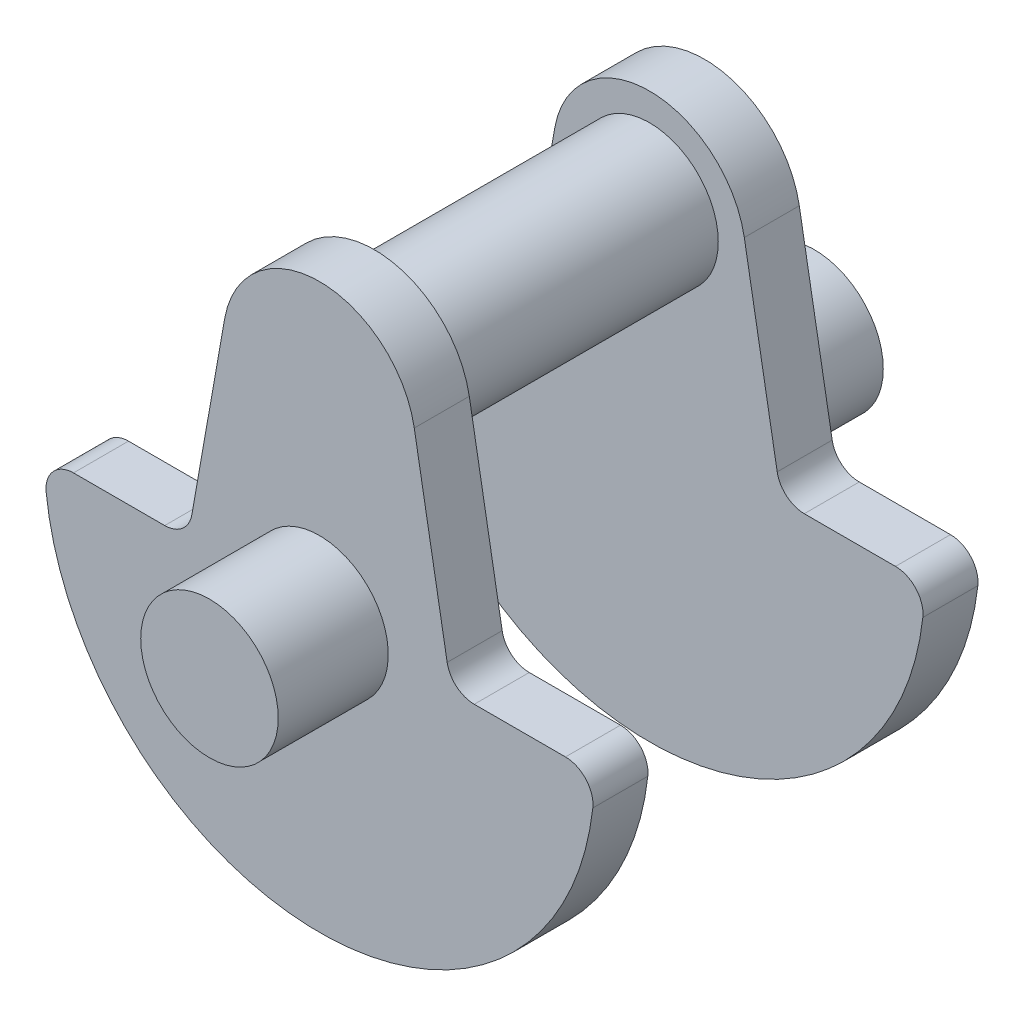
ISO-10303-21;
HEADER;
FILE_DESCRIPTION(('STEP AP214'),'2;1');
FILE_NAME('part.step','',(''),(''),'','','');
FILE_SCHEMA(('AUTOMOTIVE_DESIGN { 1 0 10303 214 1 1 1 1 }'));
ENDSEC;
DATA;
#1=APPLICATION_CONTEXT('core data for automotive mechanical design processes');
#2=APPLICATION_PROTOCOL_DEFINITION('international standard','automotive_design',2000,#1);
#3=PRODUCT_CONTEXT('',#1,'mechanical');
#4=PRODUCT('Part','Part','',(#3));
#5=PRODUCT_RELATED_PRODUCT_CATEGORY('part','',(#4));
#6=PRODUCT_DEFINITION_FORMATION('','',#4);
#7=PRODUCT_DEFINITION_CONTEXT('part definition',#1,'design');
#8=PRODUCT_DEFINITION('design','',#6,#7);
#9=PRODUCT_DEFINITION_SHAPE('','',#8);
#10=(LENGTH_UNIT() NAMED_UNIT(*) SI_UNIT(.MILLI.,.METRE.));
#11=(NAMED_UNIT(*) PLANE_ANGLE_UNIT() SI_UNIT($,.RADIAN.));
#12=(NAMED_UNIT(*) SI_UNIT($,.STERADIAN.) SOLID_ANGLE_UNIT());
#13=UNCERTAINTY_MEASURE_WITH_UNIT(LENGTH_MEASURE(1.E-05),#10,'distance_accuracy_value','');
#14=(GEOMETRIC_REPRESENTATION_CONTEXT(3) GLOBAL_UNCERTAINTY_ASSIGNED_CONTEXT((#13)) GLOBAL_UNIT_ASSIGNED_CONTEXT((#10,
#11,#12)) REPRESENTATION_CONTEXT('',''));
#15=CARTESIAN_POINT('',(0.,0.,0.));
#16=DIRECTION('',(0.,0.,1.));
#17=DIRECTION('',(1.,0.,0.));
#18=AXIS2_PLACEMENT_3D('',#15,#16,#17);
#19=CARTESIAN_POINT('',(23.2194881859126,4.09422224541768,-10.));
#20=DIRECTION('',(-0.984807753012209,-0.173648177666924,0.));
#21=DIRECTION('',(0.173648177666924,-0.984807753012209,0.));
#22=AXIS2_PLACEMENT_3D('',#19,#20,#21);
#23=PLANE('',#22);
#24=DIRECTION('',(0.173648177666924,-0.984807753012209,0.));
#25=VECTOR('',#24,1.);
#26=CARTESIAN_POINT('',(23.2194881859126,4.09422224541768,0.));
#27=LINE('',#26,#25);
#28=CARTESIAN_POINT('',(17.2341356777137,38.0388431091712,0.));
#29=VERTEX_POINT('',#28);
#30=CARTESIAN_POINT('',(23.2128694236219,4.13175911166538,0.));
#31=VERTEX_POINT('',#30);
#32=EDGE_CURVE('E156',#29,#31,#27,.T.);
#33=ORIENTED_EDGE('',*,*,#32,.T.);
#34=DIRECTION('',(0.,0.,1.));
#35=VECTOR('',#34,1.);
#36=CARTESIAN_POINT('',(23.2128694236219,4.13175911166538,-10.));
#37=LINE('',#36,#35);
#38=CARTESIAN_POINT('',(23.2128694236219,4.13175911166538,-10.));
#39=VERTEX_POINT('',#38);
#40=EDGE_CURVE('E49',#39,#31,#37,.T.);
#41=ORIENTED_EDGE('',*,*,#40,.F.);
#42=DIRECTION('',(0.173648177666924,-0.984807753012209,0.));
#43=VECTOR('',#42,1.);
#44=CARTESIAN_POINT('',(23.2194881859126,4.09422224541768,-10.));
#45=LINE('',#44,#43);
#46=CARTESIAN_POINT('',(17.2341356777137,38.0388431091712,-10.));
#47=VERTEX_POINT('',#46);
#48=EDGE_CURVE('E185',#47,#39,#45,.T.);
#49=ORIENTED_EDGE('',*,*,#48,.F.);
#50=DIRECTION('',(0.,0.,1.));
#51=VECTOR('',#50,1.);
#52=CARTESIAN_POINT('',(17.2341356777137,38.0388431091712,-10.));
#53=LINE('',#52,#51);
#54=EDGE_CURVE('E42',#47,#29,#53,.T.);
#55=ORIENTED_EDGE('',*,*,#54,.T.);
#56=EDGE_LOOP('',(#33,#41,#49,#55));
#57=FACE_BOUND('',#56,.T.);
#58=ADVANCED_FACE('F41',(#57),#23,.F.);
#59=CARTESIAN_POINT('',(28.136908188683,5.,-10.));
#60=DIRECTION('',(0.,0.,1.));
#61=DIRECTION('',(1.,0.,0.));
#62=AXIS2_PLACEMENT_3D('',#59,#60,#61);
#63=CYLINDRICAL_SURFACE('',#62,5.);
#64=CARTESIAN_POINT('',(28.136908188683,5.,0.));
#65=DIRECTION('',(0.,0.,1.));
#66=DIRECTION('',(1.,0.,0.));
#67=AXIS2_PLACEMENT_3D('',#64,#65,#66);
#68=CIRCLE('',#67,5.);
#69=CARTESIAN_POINT('',(28.136908188683,0.,0.));
#70=VERTEX_POINT('',#69);
#71=EDGE_CURVE('E95',#31,#70,#68,.T.);
#72=ORIENTED_EDGE('',*,*,#71,.T.);
#73=DIRECTION('',(0.,0.,1.));
#74=VECTOR('',#73,1.);
#75=CARTESIAN_POINT('',(28.136908188683,0.,-10.));
#76=LINE('',#75,#74);
#77=CARTESIAN_POINT('',(28.136908188683,0.,-10.));
#78=VERTEX_POINT('',#77);
#79=EDGE_CURVE('E145',#78,#70,#76,.T.);
#80=ORIENTED_EDGE('',*,*,#79,.F.);
#81=CARTESIAN_POINT('',(28.136908188683,5.,-10.));
#82=DIRECTION('',(0.,0.,1.));
#83=DIRECTION('',(1.,0.,0.));
#84=AXIS2_PLACEMENT_3D('',#81,#82,#83);
#85=CIRCLE('',#84,5.);
#86=EDGE_CURVE('E56',#39,#78,#85,.T.);
#87=ORIENTED_EDGE('',*,*,#86,.F.);
#88=ORIENTED_EDGE('',*,*,#40,.T.);
#89=EDGE_LOOP('',(#72,#80,#87,#88));
#90=FACE_BOUND('',#89,.T.);
#91=ADVANCED_FACE('F215',(#90),#63,.F.);
#92=CARTESIAN_POINT('',(0.,0.,-10.));
#93=DIRECTION('',(0.,-1.,0.));
#94=DIRECTION('',(1.,0.,0.));
#95=AXIS2_PLACEMENT_3D('',#92,#93,#94);
#96=PLANE('',#95);
#97=DIRECTION('',(1.,0.,0.));
#98=VECTOR('',#97,1.);
#99=CARTESIAN_POINT('',(0.,0.,0.));
#100=LINE('',#99,#98);
#101=CARTESIAN_POINT('',(44.7213595499958,0.,0.));
#102=VERTEX_POINT('',#101);
#103=EDGE_CURVE('E136',#70,#102,#100,.T.);
#104=ORIENTED_EDGE('',*,*,#103,.T.);
#105=DIRECTION('',(0.,0.,1.));
#106=VECTOR('',#105,1.);
#107=CARTESIAN_POINT('',(44.7213595499958,0.,-10.));
#108=LINE('',#107,#106);
#109=CARTESIAN_POINT('',(44.7213595499958,0.,-10.));
#110=VERTEX_POINT('',#109);
#111=EDGE_CURVE('E137',#110,#102,#108,.T.);
#112=ORIENTED_EDGE('',*,*,#111,.F.);
#113=DIRECTION('',(1.,0.,0.));
#114=VECTOR('',#113,1.);
#115=CARTESIAN_POINT('',(0.,0.,-10.));
#116=LINE('',#115,#114);
#117=EDGE_CURVE('E126',#78,#110,#116,.T.);
#118=ORIENTED_EDGE('',*,*,#117,.F.);
#119=ORIENTED_EDGE('',*,*,#79,.T.);
#120=EDGE_LOOP('',(#104,#112,#118,#119));
#121=FACE_BOUND('',#120,.T.);
#122=ADVANCED_FACE('F140',(#121),#96,.F.);
#123=CARTESIAN_POINT('',(44.7213595499958,-5.,-10.));
#124=DIRECTION('',(0.,0.,1.));
#125=DIRECTION('',(1.,0.,0.));
#126=AXIS2_PLACEMENT_3D('',#123,#124,#125);
#127=CYLINDRICAL_SURFACE('',#126,5.);
#128=CARTESIAN_POINT('',(44.7213595499958,-5.,0.));
#129=DIRECTION('',(0.,0.,1.));
#130=DIRECTION('',(1.,0.,0.));
#131=AXIS2_PLACEMENT_3D('',#128,#129,#130);
#132=CIRCLE('',#131,5.);
#133=CARTESIAN_POINT('',(49.6903994999953,-5.55555555555555,0.));
#134=VERTEX_POINT('',#133);
#135=EDGE_CURVE('E177',#102,#134,#132,.F.);
#136=ORIENTED_EDGE('',*,*,#135,.T.);
#137=DIRECTION('',(0.,0.,1.));
#138=VECTOR('',#137,1.);
#139=CARTESIAN_POINT('',(49.6903994999953,-5.55555555555555,-10.));
#140=LINE('',#139,#138);
#141=CARTESIAN_POINT('',(49.6903994999953,-5.55555555555555,-10.));
#142=VERTEX_POINT('',#141);
#143=EDGE_CURVE('E144',#142,#134,#140,.T.);
#144=ORIENTED_EDGE('',*,*,#143,.F.);
#145=CARTESIAN_POINT('',(44.7213595499958,-5.,-10.));
#146=DIRECTION('',(0.,0.,1.));
#147=DIRECTION('',(1.,0.,0.));
#148=AXIS2_PLACEMENT_3D('',#145,#146,#147);
#149=CIRCLE('',#148,5.);
#150=EDGE_CURVE('E133',#110,#142,#149,.F.);
#151=ORIENTED_EDGE('',*,*,#150,.F.);
#152=ORIENTED_EDGE('',*,*,#111,.T.);
#153=EDGE_LOOP('',(#136,#144,#151,#152));
#154=FACE_BOUND('',#153,.T.);
#155=ADVANCED_FACE('F150',(#154),#127,.T.);
#156=CARTESIAN_POINT('',(0.,0.,-10.));
#157=DIRECTION('',(0.,0.,1.));
#158=DIRECTION('',(1.,0.,0.));
#159=AXIS2_PLACEMENT_3D('',#156,#157,#158);
#160=CYLINDRICAL_SURFACE('',#159,50.);
#161=CARTESIAN_POINT('',(0.,0.,0.));
#162=DIRECTION('',(0.,0.,1.));
#163=DIRECTION('',(1.,0.,0.));
#164=AXIS2_PLACEMENT_3D('',#161,#162,#163);
#165=CIRCLE('',#164,50.);
#166=CARTESIAN_POINT('',(-49.6903994999953,-5.55555555555555,0.));
#167=VERTEX_POINT('',#166);
#168=EDGE_CURVE('E171',#167,#134,#165,.T.);
#169=ORIENTED_EDGE('',*,*,#168,.F.);
#170=DIRECTION('',(0.,0.,1.));
#171=VECTOR('',#170,1.);
#172=CARTESIAN_POINT('',(-49.6903994999953,-5.55555555555555,-10.));
#173=LINE('',#172,#171);
#174=CARTESIAN_POINT('',(-49.6903994999953,-5.55555555555555,-10.));
#175=VERTEX_POINT('',#174);
#176=EDGE_CURVE('E187',#175,#167,#173,.T.);
#177=ORIENTED_EDGE('',*,*,#176,.F.);
#178=CARTESIAN_POINT('',(0.,0.,-10.));
#179=DIRECTION('',(0.,0.,1.));
#180=DIRECTION('',(1.,0.,0.));
#181=AXIS2_PLACEMENT_3D('',#178,#179,#180);
#182=CIRCLE('',#181,50.);
#183=EDGE_CURVE('E149',#175,#142,#182,.T.);
#184=ORIENTED_EDGE('',*,*,#183,.T.);
#185=ORIENTED_EDGE('',*,*,#143,.T.);
#186=EDGE_LOOP('',(#169,#177,#184,#185));
#187=FACE_BOUND('',#186,.T.);
#188=ADVANCED_FACE('F223',(#187),#160,.T.);
#189=CARTESIAN_POINT('',(-44.7213595499958,-5.,-10.));
#190=DIRECTION('',(0.,0.,1.));
#191=DIRECTION('',(1.,0.,0.));
#192=AXIS2_PLACEMENT_3D('',#189,#190,#191);
#193=CYLINDRICAL_SURFACE('',#192,5.);
#194=CARTESIAN_POINT('',(-44.7213595499958,-5.,0.));
#195=DIRECTION('',(0.,0.,1.));
#196=DIRECTION('',(1.,0.,0.));
#197=AXIS2_PLACEMENT_3D('',#194,#195,#196);
#198=CIRCLE('',#197,5.);
#199=CARTESIAN_POINT('',(-44.7213595499958,0.,0.));
#200=VERTEX_POINT('',#199);
#201=EDGE_CURVE('E175',#200,#167,#198,.T.);
#202=ORIENTED_EDGE('',*,*,#201,.F.);
#203=DIRECTION('',(0.,0.,1.));
#204=VECTOR('',#203,1.);
#205=CARTESIAN_POINT('',(-44.7213595499958,0.,-10.));
#206=LINE('',#205,#204);
#207=CARTESIAN_POINT('',(-44.7213595499958,0.,-10.));
#208=VERTEX_POINT('',#207);
#209=EDGE_CURVE('E188',#208,#200,#206,.T.);
#210=ORIENTED_EDGE('',*,*,#209,.F.);
#211=CARTESIAN_POINT('',(-44.7213595499958,-5.,-10.));
#212=DIRECTION('',(0.,0.,1.));
#213=DIRECTION('',(1.,0.,0.));
#214=AXIS2_PLACEMENT_3D('',#211,#212,#213);
#215=CIRCLE('',#214,5.);
#216=EDGE_CURVE('E151',#208,#175,#215,.T.);
#217=ORIENTED_EDGE('',*,*,#216,.T.);
#218=ORIENTED_EDGE('',*,*,#176,.T.);
#219=EDGE_LOOP('',(#202,#210,#217,#218));
#220=FACE_BOUND('',#219,.T.);
#221=ADVANCED_FACE('F228',(#220),#193,.T.);
#222=CARTESIAN_POINT('',(0.,0.,-10.));
#223=DIRECTION('',(0.,-1.,0.));
#224=DIRECTION('',(1.,0.,0.));
#225=AXIS2_PLACEMENT_3D('',#222,#223,#224);
#226=PLANE('',#225);
#227=DIRECTION('',(1.,0.,0.));
#228=VECTOR('',#227,1.);
#229=CARTESIAN_POINT('',(0.,0.,0.));
#230=LINE('',#229,#228);
#231=CARTESIAN_POINT('',(-28.136908188683,0.,0.));
#232=VERTEX_POINT('',#231);
#233=EDGE_CURVE('E166',#200,#232,#230,.T.);
#234=ORIENTED_EDGE('',*,*,#233,.T.);
#235=DIRECTION('',(0.,0.,1.));
#236=VECTOR('',#235,1.);
#237=CARTESIAN_POINT('',(-28.136908188683,0.,-10.));
#238=LINE('',#237,#236);
#239=CARTESIAN_POINT('',(-28.136908188683,0.,-10.));
#240=VERTEX_POINT('',#239);
#241=EDGE_CURVE('E186',#240,#232,#238,.T.);
#242=ORIENTED_EDGE('',*,*,#241,.F.);
#243=DIRECTION('',(1.,0.,0.));
#244=VECTOR('',#243,1.);
#245=CARTESIAN_POINT('',(0.,0.,-10.));
#246=LINE('',#245,#244);
#247=EDGE_CURVE('E252',#208,#240,#246,.T.);
#248=ORIENTED_EDGE('',*,*,#247,.F.);
#249=ORIENTED_EDGE('',*,*,#209,.T.);
#250=EDGE_LOOP('',(#234,#242,#248,#249));
#251=FACE_BOUND('',#250,.T.);
#252=ADVANCED_FACE('F234',(#251),#226,.F.);
#253=CARTESIAN_POINT('',(-28.136908188683,5.,-10.));
#254=DIRECTION('',(0.,0.,1.));
#255=DIRECTION('',(1.,0.,0.));
#256=AXIS2_PLACEMENT_3D('',#253,#254,#255);
#257=CYLINDRICAL_SURFACE('',#256,5.);
#258=CARTESIAN_POINT('',(-28.136908188683,5.,0.));
#259=DIRECTION('',(0.,0.,1.));
#260=DIRECTION('',(1.,0.,0.));
#261=AXIS2_PLACEMENT_3D('',#258,#259,#260);
#262=CIRCLE('',#261,5.);
#263=CARTESIAN_POINT('',(-23.2128694236219,4.13175911166538,0.));
#264=VERTEX_POINT('',#263);
#265=EDGE_CURVE('E167',#264,#232,#262,.F.);
#266=ORIENTED_EDGE('',*,*,#265,.F.);
#267=DIRECTION('',(0.,0.,1.));
#268=VECTOR('',#267,1.);
#269=CARTESIAN_POINT('',(-23.2128694236219,4.13175911166538,-10.));
#270=LINE('',#269,#268);
#271=CARTESIAN_POINT('',(-23.2128694236219,4.13175911166538,-10.));
#272=VERTEX_POINT('',#271);
#273=EDGE_CURVE('E194',#272,#264,#270,.T.);
#274=ORIENTED_EDGE('',*,*,#273,.F.);
#275=CARTESIAN_POINT('',(-28.136908188683,5.,-10.));
#276=DIRECTION('',(0.,0.,1.));
#277=DIRECTION('',(1.,0.,0.));
#278=AXIS2_PLACEMENT_3D('',#275,#276,#277);
#279=CIRCLE('',#278,5.);
#280=EDGE_CURVE('E250',#272,#240,#279,.F.);
#281=ORIENTED_EDGE('',*,*,#280,.T.);
#282=ORIENTED_EDGE('',*,*,#241,.T.);
#283=EDGE_LOOP('',(#266,#274,#281,#282));
#284=FACE_BOUND('',#283,.T.);
#285=ADVANCED_FACE('F208',(#284),#257,.F.);
#286=CARTESIAN_POINT('',(-23.2194881859126,4.09422224541768,-10.));
#287=DIRECTION('',(-0.984807753012209,0.173648177666924,0.));
#288=DIRECTION('',(-0.173648177666924,-0.984807753012209,0.));
#289=AXIS2_PLACEMENT_3D('',#286,#287,#288);
#290=PLANE('',#289);
#291=DIRECTION('',(-0.173648177666924,-0.984807753012209,0.));
#292=VECTOR('',#291,1.);
#293=CARTESIAN_POINT('',(-23.2194881859126,4.09422224541768,0.));
#294=LINE('',#293,#292);
#295=CARTESIAN_POINT('',(-17.2341356777137,38.0388431091712,0.));
#296=VERTEX_POINT('',#295);
#297=EDGE_CURVE('E162',#296,#264,#294,.T.);
#298=ORIENTED_EDGE('',*,*,#297,.F.);
#299=DIRECTION('',(0.,0.,1.));
#300=VECTOR('',#299,1.);
#301=CARTESIAN_POINT('',(-17.2341356777137,38.0388431091712,-10.));
#302=LINE('',#301,#300);
#303=CARTESIAN_POINT('',(-17.2341356777137,38.0388431091712,-10.));
#304=VERTEX_POINT('',#303);
#305=EDGE_CURVE('E192',#304,#296,#302,.T.);
#306=ORIENTED_EDGE('',*,*,#305,.F.);
#307=DIRECTION('',(-0.173648177666924,-0.984807753012209,0.));
#308=VECTOR('',#307,1.);
#309=CARTESIAN_POINT('',(-23.2194881859126,4.09422224541768,-10.));
#310=LINE('',#309,#308);
#311=EDGE_CURVE('E247',#304,#272,#310,.T.);
#312=ORIENTED_EDGE('',*,*,#311,.T.);
#313=ORIENTED_EDGE('',*,*,#273,.T.);
#314=EDGE_LOOP('',(#298,#306,#312,#313));
#315=FACE_BOUND('',#314,.T.);
#316=ADVANCED_FACE('F203',(#315),#290,.T.);
#317=CARTESIAN_POINT('',(0.,35.,-10.));
#318=DIRECTION('',(0.,0.,1.));
#319=DIRECTION('',(1.,0.,0.));
#320=AXIS2_PLACEMENT_3D('',#317,#318,#319);
#321=CYLINDRICAL_SURFACE('',#320,17.5);
#322=CARTESIAN_POINT('',(0.,35.,0.));
#323=DIRECTION('',(0.,0.,1.));
#324=DIRECTION('',(1.,0.,0.));
#325=AXIS2_PLACEMENT_3D('',#322,#323,#324);
#326=CIRCLE('',#325,17.5);
#327=EDGE_CURVE('E157',#29,#296,#326,.T.);
#328=ORIENTED_EDGE('',*,*,#327,.F.);
#329=ORIENTED_EDGE('',*,*,#54,.F.);
#330=CARTESIAN_POINT('',(0.,35.,-10.));
#331=DIRECTION('',(0.,0.,1.));
#332=DIRECTION('',(1.,0.,0.));
#333=AXIS2_PLACEMENT_3D('',#330,#331,#332);
#334=CIRCLE('',#333,17.5);
#335=EDGE_CURVE('E246',#47,#304,#334,.T.);
#336=ORIENTED_EDGE('',*,*,#335,.T.);
#337=ORIENTED_EDGE('',*,*,#305,.T.);
#338=EDGE_LOOP('',(#328,#329,#336,#337));
#339=FACE_BOUND('',#338,.T.);
#340=ADVANCED_FACE('F200',(#339),#321,.T.);
#341=CARTESIAN_POINT('',(0.,0.,-10.));
#342=DIRECTION('',(0.,0.,1.));
#343=DIRECTION('',(1.,0.,0.));
#344=AXIS2_PLACEMENT_3D('',#341,#342,#343);
#345=PLANE('',#344);
#346=CARTESIAN_POINT('',(0.,0.,-10.));
#347=DIRECTION('',(0.,0.,1.));
#348=DIRECTION('',(1.,0.,0.));
#349=AXIS2_PLACEMENT_3D('',#346,#347,#348);
#350=CIRCLE('',#349,12.5);
#351=CARTESIAN_POINT('',(12.5,0.,-10.));
#352=VERTEX_POINT('',#351);
#353=EDGE_CURVE('E159',#352,#352,#350,.T.);
#354=ORIENTED_EDGE('',*,*,#353,.T.);
#355=EDGE_LOOP('',(#354));
#356=FACE_BOUND('',#355,.T.);
#357=ORIENTED_EDGE('',*,*,#48,.T.);
#358=ORIENTED_EDGE('',*,*,#86,.T.);
#359=ORIENTED_EDGE('',*,*,#117,.T.);
#360=ORIENTED_EDGE('',*,*,#150,.T.);
#361=ORIENTED_EDGE('',*,*,#183,.F.);
#362=ORIENTED_EDGE('',*,*,#216,.F.);
#363=ORIENTED_EDGE('',*,*,#247,.T.);
#364=ORIENTED_EDGE('',*,*,#280,.F.);
#365=ORIENTED_EDGE('',*,*,#311,.F.);
#366=ORIENTED_EDGE('',*,*,#335,.F.);
#367=EDGE_LOOP('',(#357,#358,#359,#360,#361,#362,#363,#364,#365,#366));
#368=FACE_BOUND('',#367,.T.);
#369=ADVANCED_FACE('F128',(#356,#368),#345,.F.);
#370=CARTESIAN_POINT('',(0.,0.,0.));
#371=DIRECTION('',(0.,0.,1.));
#372=DIRECTION('',(1.,0.,0.));
#373=AXIS2_PLACEMENT_3D('',#370,#371,#372);
#374=PLANE('',#373);
#375=CARTESIAN_POINT('',(0.,35.,0.));
#376=DIRECTION('',(0.,0.,1.));
#377=DIRECTION('',(1.,0.,0.));
#378=AXIS2_PLACEMENT_3D('',#375,#376,#377);
#379=CIRCLE('',#378,12.5);
#380=CARTESIAN_POINT('',(12.5,35.,0.));
#381=VERTEX_POINT('',#380);
#382=EDGE_CURVE('E267',#381,#381,#379,.T.);
#383=ORIENTED_EDGE('',*,*,#382,.F.);
#384=EDGE_LOOP('',(#383));
#385=FACE_BOUND('',#384,.T.);
#386=ORIENTED_EDGE('',*,*,#32,.F.);
#387=ORIENTED_EDGE('',*,*,#327,.T.);
#388=ORIENTED_EDGE('',*,*,#297,.T.);
#389=ORIENTED_EDGE('',*,*,#265,.T.);
#390=ORIENTED_EDGE('',*,*,#233,.F.);
#391=ORIENTED_EDGE('',*,*,#201,.T.);
#392=ORIENTED_EDGE('',*,*,#168,.T.);
#393=ORIENTED_EDGE('',*,*,#135,.F.);
#394=ORIENTED_EDGE('',*,*,#103,.F.);
#395=ORIENTED_EDGE('',*,*,#71,.F.);
#396=EDGE_LOOP('',(#386,#387,#388,#389,#390,#391,#392,#393,#394,#395));
#397=FACE_BOUND('',#396,.T.);
#398=ADVANCED_FACE('F196',(#385,#397),#374,.T.);
#399=CARTESIAN_POINT('',(0.,0.,-30.));
#400=DIRECTION('',(0.,0.,1.));
#401=DIRECTION('',(1.,0.,0.));
#402=AXIS2_PLACEMENT_3D('',#399,#400,#401);
#403=CYLINDRICAL_SURFACE('',#402,12.5);
#404=CARTESIAN_POINT('',(0.,0.,-30.));
#405=DIRECTION('',(0.,0.,1.));
#406=DIRECTION('',(1.,0.,0.));
#407=AXIS2_PLACEMENT_3D('',#404,#405,#406);
#408=CIRCLE('',#407,12.5);
#409=CARTESIAN_POINT('',(12.5,0.,-30.));
#410=VERTEX_POINT('',#409);
#411=EDGE_CURVE('E264',#410,#410,#408,.T.);
#412=ORIENTED_EDGE('',*,*,#411,.T.);
#413=EDGE_LOOP('',(#412));
#414=FACE_BOUND('',#413,.T.);
#415=ORIENTED_EDGE('',*,*,#353,.F.);
#416=EDGE_LOOP('',(#415));
#417=FACE_BOUND('',#416,.T.);
#418=ADVANCED_FACE('F487',(#414,#417),#403,.T.);
#419=CARTESIAN_POINT('',(0.,0.,-30.));
#420=DIRECTION('',(0.,0.,1.));
#421=DIRECTION('',(1.,0.,0.));
#422=AXIS2_PLACEMENT_3D('',#419,#420,#421);
#423=PLANE('',#422);
#424=ORIENTED_EDGE('',*,*,#411,.F.);
#425=EDGE_LOOP('',(#424));
#426=FACE_BOUND('',#425,.T.);
#427=ADVANCED_FACE('F484',(#426),#423,.F.);
#428=CARTESIAN_POINT('',(0.,35.,50.));
#429=DIRECTION('',(0.,0.,-1.));
#430=DIRECTION('',(-1.,0.,0.));
#431=AXIS2_PLACEMENT_3D('',#428,#429,#430);
#432=CYLINDRICAL_SURFACE('',#431,12.5);
#433=CARTESIAN_POINT('',(0.,35.,50.));
#434=DIRECTION('',(0.,0.,1.));
#435=DIRECTION('',(1.,0.,0.));
#436=AXIS2_PLACEMENT_3D('',#433,#434,#435);
#437=CIRCLE('',#436,12.5);
#438=CARTESIAN_POINT('',(12.5,35.,50.));
#439=VERTEX_POINT('',#438);
#440=EDGE_CURVE('E268',#439,#439,#437,.T.);
#441=ORIENTED_EDGE('',*,*,#440,.F.);
#442=EDGE_LOOP('',(#441));
#443=FACE_BOUND('',#442,.T.);
#444=ORIENTED_EDGE('',*,*,#382,.T.);
#445=EDGE_LOOP('',(#444));
#446=FACE_BOUND('',#445,.T.);
#447=ADVANCED_FACE('F485',(#443,#446),#432,.T.);
#448=CARTESIAN_POINT('',(23.2194881859126,4.09422224541768,60.));
#449=DIRECTION('',(0.984807753012209,0.173648177666924,0.));
#450=DIRECTION('',(-0.173648177666924,0.984807753012209,0.));
#451=AXIS2_PLACEMENT_3D('',#448,#449,#450);
#452=PLANE('',#451);
#453=DIRECTION('',(0.173648177666924,-0.984807753012209,0.));
#454=VECTOR('',#453,1.);
#455=CARTESIAN_POINT('',(23.2194881859126,4.09422224541768,50.));
#456=LINE('',#455,#454);
#457=CARTESIAN_POINT('',(17.2341356777137,38.0388431091712,50.));
#458=VERTEX_POINT('',#457);
#459=CARTESIAN_POINT('',(23.2128694236219,4.13175911166538,50.));
#460=VERTEX_POINT('',#459);
#461=EDGE_CURVE('E334',#458,#460,#456,.T.);
#462=ORIENTED_EDGE('',*,*,#461,.F.);
#463=DIRECTION('',(0.,0.,-1.));
#464=VECTOR('',#463,1.);
#465=CARTESIAN_POINT('',(17.2341356777137,38.0388431091712,60.));
#466=LINE('',#465,#464);
#467=CARTESIAN_POINT('',(17.2341356777137,38.0388431091712,60.));
#468=VERTEX_POINT('',#467);
#469=EDGE_CURVE('E275',#468,#458,#466,.T.);
#470=ORIENTED_EDGE('',*,*,#469,.F.);
#471=DIRECTION('',(0.173648177666924,-0.984807753012209,0.));
#472=VECTOR('',#471,1.);
#473=CARTESIAN_POINT('',(23.2194881859126,4.09422224541768,60.));
#474=LINE('',#473,#472);
#475=CARTESIAN_POINT('',(23.2128694236219,4.13175911166538,60.));
#476=VERTEX_POINT('',#475);
#477=EDGE_CURVE('E306',#468,#476,#474,.T.);
#478=ORIENTED_EDGE('',*,*,#477,.T.);
#479=DIRECTION('',(0.,0.,-1.));
#480=VECTOR('',#479,1.);
#481=CARTESIAN_POINT('',(23.2128694236219,4.13175911166538,60.));
#482=LINE('',#481,#480);
#483=EDGE_CURVE('E274',#476,#460,#482,.T.);
#484=ORIENTED_EDGE('',*,*,#483,.T.);
#485=EDGE_LOOP('',(#462,#470,#478,#484));
#486=FACE_BOUND('',#485,.T.);
#487=ADVANCED_FACE('F393',(#486),#452,.T.);
#488=CARTESIAN_POINT('',(0.,35.,60.));
#489=DIRECTION('',(0.,0.,-1.));
#490=DIRECTION('',(-1.,0.,0.));
#491=AXIS2_PLACEMENT_3D('',#488,#489,#490);
#492=CYLINDRICAL_SURFACE('',#491,17.5);
#493=CARTESIAN_POINT('',(0.,35.,50.));
#494=DIRECTION('',(0.,0.,1.));
#495=DIRECTION('',(1.,0.,0.));
#496=AXIS2_PLACEMENT_3D('',#493,#494,#495);
#497=CIRCLE('',#496,17.5);
#498=CARTESIAN_POINT('',(-17.2341356777137,38.0388431091712,50.));
#499=VERTEX_POINT('',#498);
#500=EDGE_CURVE('E301',#458,#499,#497,.T.);
#501=ORIENTED_EDGE('',*,*,#500,.T.);
#502=DIRECTION('',(0.,0.,-1.));
#503=VECTOR('',#502,1.);
#504=CARTESIAN_POINT('',(-17.2341356777137,38.0388431091712,60.));
#505=LINE('',#504,#503);
#506=CARTESIAN_POINT('',(-17.2341356777137,38.0388431091712,60.));
#507=VERTEX_POINT('',#506);
#508=EDGE_CURVE('E296',#507,#499,#505,.T.);
#509=ORIENTED_EDGE('',*,*,#508,.F.);
#510=CARTESIAN_POINT('',(0.,35.,60.));
#511=DIRECTION('',(0.,0.,1.));
#512=DIRECTION('',(1.,0.,0.));
#513=AXIS2_PLACEMENT_3D('',#510,#511,#512);
#514=CIRCLE('',#513,17.5);
#515=EDGE_CURVE('E276',#468,#507,#514,.T.);
#516=ORIENTED_EDGE('',*,*,#515,.F.);
#517=ORIENTED_EDGE('',*,*,#469,.T.);
#518=EDGE_LOOP('',(#501,#509,#516,#517));
#519=FACE_BOUND('',#518,.T.);
#520=ADVANCED_FACE('F434',(#519),#492,.T.);
#521=CARTESIAN_POINT('',(-23.2194881859126,4.09422224541768,60.));
#522=DIRECTION('',(0.984807753012209,-0.173648177666924,0.));
#523=DIRECTION('',(0.173648177666924,0.984807753012209,0.));
#524=AXIS2_PLACEMENT_3D('',#521,#522,#523);
#525=PLANE('',#524);
#526=DIRECTION('',(-0.173648177666924,-0.984807753012209,0.));
#527=VECTOR('',#526,1.);
#528=CARTESIAN_POINT('',(-23.2194881859126,4.09422224541768,50.));
#529=LINE('',#528,#527);
#530=CARTESIAN_POINT('',(-23.2128694236219,4.13175911166538,50.));
#531=VERTEX_POINT('',#530);
#532=EDGE_CURVE('E310',#499,#531,#529,.T.);
#533=ORIENTED_EDGE('',*,*,#532,.T.);
#534=DIRECTION('',(0.,0.,-1.));
#535=VECTOR('',#534,1.);
#536=CARTESIAN_POINT('',(-23.2128694236219,4.13175911166538,60.));
#537=LINE('',#536,#535);
#538=CARTESIAN_POINT('',(-23.2128694236219,4.13175911166538,60.));
#539=VERTEX_POINT('',#538);
#540=EDGE_CURVE('E300',#539,#531,#537,.T.);
#541=ORIENTED_EDGE('',*,*,#540,.F.);
#542=DIRECTION('',(-0.173648177666924,-0.984807753012209,0.));
#543=VECTOR('',#542,1.);
#544=CARTESIAN_POINT('',(-23.2194881859126,4.09422224541768,60.));
#545=LINE('',#544,#543);
#546=EDGE_CURVE('E339',#507,#539,#545,.T.);
#547=ORIENTED_EDGE('',*,*,#546,.F.);
#548=ORIENTED_EDGE('',*,*,#508,.T.);
#549=EDGE_LOOP('',(#533,#541,#547,#548));
#550=FACE_BOUND('',#549,.T.);
#551=ADVANCED_FACE('F439',(#550),#525,.F.);
#552=CARTESIAN_POINT('',(-28.136908188683,5.,60.));
#553=DIRECTION('',(0.,0.,-1.));
#554=DIRECTION('',(-1.,0.,0.));
#555=AXIS2_PLACEMENT_3D('',#552,#553,#554);
#556=CYLINDRICAL_SURFACE('',#555,5.);
#557=CARTESIAN_POINT('',(-28.136908188683,5.,50.));
#558=DIRECTION('',(0.,0.,1.));
#559=DIRECTION('',(1.,0.,0.));
#560=AXIS2_PLACEMENT_3D('',#557,#558,#559);
#561=CIRCLE('',#560,5.);
#562=CARTESIAN_POINT('',(-28.136908188683,0.,50.));
#563=VERTEX_POINT('',#562);
#564=EDGE_CURVE('E315',#531,#563,#561,.F.);
#565=ORIENTED_EDGE('',*,*,#564,.T.);
#566=DIRECTION('',(0.,0.,-1.));
#567=VECTOR('',#566,1.);
#568=CARTESIAN_POINT('',(-28.136908188683,0.,60.));
#569=LINE('',#568,#567);
#570=CARTESIAN_POINT('',(-28.136908188683,0.,60.));
#571=VERTEX_POINT('',#570);
#572=EDGE_CURVE('E294',#571,#563,#569,.T.);
#573=ORIENTED_EDGE('',*,*,#572,.F.);
#574=CARTESIAN_POINT('',(-28.136908188683,5.,60.));
#575=DIRECTION('',(0.,0.,1.));
#576=DIRECTION('',(1.,0.,0.));
#577=AXIS2_PLACEMENT_3D('',#574,#575,#576);
#578=CIRCLE('',#577,5.);
#579=EDGE_CURVE('E344',#539,#571,#578,.F.);
#580=ORIENTED_EDGE('',*,*,#579,.F.);
#581=ORIENTED_EDGE('',*,*,#540,.T.);
#582=EDGE_LOOP('',(#565,#573,#580,#581));
#583=FACE_BOUND('',#582,.T.);
#584=ADVANCED_FACE('F450',(#583),#556,.F.);
#585=CARTESIAN_POINT('',(0.,0.,60.));
#586=DIRECTION('',(0.,1.,0.));
#587=DIRECTION('',(-1.,0.,0.));
#588=AXIS2_PLACEMENT_3D('',#585,#586,#587);
#589=PLANE('',#588);
#590=DIRECTION('',(1.,0.,0.));
#591=VECTOR('',#590,1.);
#592=CARTESIAN_POINT('',(0.,0.,50.));
#593=LINE('',#592,#591);
#594=CARTESIAN_POINT('',(-44.7213595499958,0.,50.));
#595=VERTEX_POINT('',#594);
#596=EDGE_CURVE('E312',#595,#563,#593,.T.);
#597=ORIENTED_EDGE('',*,*,#596,.F.);
#598=DIRECTION('',(0.,0.,-1.));
#599=VECTOR('',#598,1.);
#600=CARTESIAN_POINT('',(-44.7213595499958,0.,60.));
#601=LINE('',#600,#599);
#602=CARTESIAN_POINT('',(-44.7213595499958,0.,60.));
#603=VERTEX_POINT('',#602);
#604=EDGE_CURVE('E292',#603,#595,#601,.T.);
#605=ORIENTED_EDGE('',*,*,#604,.F.);
#606=DIRECTION('',(1.,0.,0.));
#607=VECTOR('',#606,1.);
#608=CARTESIAN_POINT('',(0.,0.,60.));
#609=LINE('',#608,#607);
#610=EDGE_CURVE('E341',#603,#571,#609,.T.);
#611=ORIENTED_EDGE('',*,*,#610,.T.);
#612=ORIENTED_EDGE('',*,*,#572,.T.);
#613=EDGE_LOOP('',(#597,#605,#611,#612));
#614=FACE_BOUND('',#613,.T.);
#615=ADVANCED_FACE('F452',(#614),#589,.T.);
#616=CARTESIAN_POINT('',(-44.7213595499958,-5.,60.));
#617=DIRECTION('',(0.,0.,-1.));
#618=DIRECTION('',(-1.,0.,0.));
#619=AXIS2_PLACEMENT_3D('',#616,#617,#618);
#620=CYLINDRICAL_SURFACE('',#619,5.);
#621=CARTESIAN_POINT('',(-44.7213595499958,-5.,50.));
#622=DIRECTION('',(0.,0.,1.));
#623=DIRECTION('',(1.,0.,0.));
#624=AXIS2_PLACEMENT_3D('',#621,#622,#623);
#625=CIRCLE('',#624,5.);
#626=CARTESIAN_POINT('',(-49.6903994999953,-5.55555555555555,50.));
#627=VERTEX_POINT('',#626);
#628=EDGE_CURVE('E318',#595,#627,#625,.T.);
#629=ORIENTED_EDGE('',*,*,#628,.T.);
#630=DIRECTION('',(0.,0.,-1.));
#631=VECTOR('',#630,1.);
#632=CARTESIAN_POINT('',(-49.6903994999953,-5.55555555555555,60.));
#633=LINE('',#632,#631);
#634=CARTESIAN_POINT('',(-49.6903994999953,-5.55555555555555,60.));
#635=VERTEX_POINT('',#634);
#636=EDGE_CURVE('E287',#635,#627,#633,.T.);
#637=ORIENTED_EDGE('',*,*,#636,.F.);
#638=CARTESIAN_POINT('',(-44.7213595499958,-5.,60.));
#639=DIRECTION('',(0.,0.,1.));
#640=DIRECTION('',(1.,0.,0.));
#641=AXIS2_PLACEMENT_3D('',#638,#639,#640);
#642=CIRCLE('',#641,5.);
#643=EDGE_CURVE('E346',#603,#635,#642,.T.);
#644=ORIENTED_EDGE('',*,*,#643,.F.);
#645=ORIENTED_EDGE('',*,*,#604,.T.);
#646=EDGE_LOOP('',(#629,#637,#644,#645));
#647=FACE_BOUND('',#646,.T.);
#648=ADVANCED_FACE('F451',(#647),#620,.T.);
#649=CARTESIAN_POINT('',(0.,0.,60.));
#650=DIRECTION('',(0.,0.,-1.));
#651=DIRECTION('',(-1.,0.,0.));
#652=AXIS2_PLACEMENT_3D('',#649,#650,#651);
#653=CYLINDRICAL_SURFACE('',#652,50.);
#654=CARTESIAN_POINT('',(0.,0.,50.));
#655=DIRECTION('',(0.,0.,1.));
#656=DIRECTION('',(1.,0.,0.));
#657=AXIS2_PLACEMENT_3D('',#654,#655,#656);
#658=CIRCLE('',#657,50.);
#659=CARTESIAN_POINT('',(49.6903994999953,-5.55555555555555,50.));
#660=VERTEX_POINT('',#659);
#661=EDGE_CURVE('E321',#627,#660,#658,.T.);
#662=ORIENTED_EDGE('',*,*,#661,.T.);
#663=DIRECTION('',(0.,0.,-1.));
#664=VECTOR('',#663,1.);
#665=CARTESIAN_POINT('',(49.6903994999953,-5.55555555555555,60.));
#666=LINE('',#665,#664);
#667=CARTESIAN_POINT('',(49.6903994999953,-5.55555555555555,60.));
#668=VERTEX_POINT('',#667);
#669=EDGE_CURVE('E281',#668,#660,#666,.T.);
#670=ORIENTED_EDGE('',*,*,#669,.F.);
#671=CARTESIAN_POINT('',(0.,0.,60.));
#672=DIRECTION('',(0.,0.,1.));
#673=DIRECTION('',(1.,0.,0.));
#674=AXIS2_PLACEMENT_3D('',#671,#672,#673);
#675=CIRCLE('',#674,50.);
#676=EDGE_CURVE('E352',#635,#668,#675,.T.);
#677=ORIENTED_EDGE('',*,*,#676,.F.);
#678=ORIENTED_EDGE('',*,*,#636,.T.);
#679=EDGE_LOOP('',(#662,#670,#677,#678));
#680=FACE_BOUND('',#679,.T.);
#681=ADVANCED_FACE('F458',(#680),#653,.T.);
#682=CARTESIAN_POINT('',(44.7213595499958,-5.,60.));
#683=DIRECTION('',(0.,0.,-1.));
#684=DIRECTION('',(-1.,0.,0.));
#685=AXIS2_PLACEMENT_3D('',#682,#683,#684);
#686=CYLINDRICAL_SURFACE('',#685,5.);
#687=CARTESIAN_POINT('',(44.7213595499958,-5.,50.));
#688=DIRECTION('',(0.,0.,1.));
#689=DIRECTION('',(1.,0.,0.));
#690=AXIS2_PLACEMENT_3D('',#687,#688,#689);
#691=CIRCLE('',#690,5.);
#692=CARTESIAN_POINT('',(44.7213595499958,0.,50.));
#693=VERTEX_POINT('',#692);
#694=EDGE_CURVE('E322',#693,#660,#691,.F.);
#695=ORIENTED_EDGE('',*,*,#694,.F.);
#696=DIRECTION('',(0.,0.,-1.));
#697=VECTOR('',#696,1.);
#698=CARTESIAN_POINT('',(44.7213595499958,0.,60.));
#699=LINE('',#698,#697);
#700=CARTESIAN_POINT('',(44.7213595499958,0.,60.));
#701=VERTEX_POINT('',#700);
#702=EDGE_CURVE('E285',#701,#693,#699,.T.);
#703=ORIENTED_EDGE('',*,*,#702,.F.);
#704=CARTESIAN_POINT('',(44.7213595499958,-5.,60.));
#705=DIRECTION('',(0.,0.,1.));
#706=DIRECTION('',(1.,0.,0.));
#707=AXIS2_PLACEMENT_3D('',#704,#705,#706);
#708=CIRCLE('',#707,5.);
#709=EDGE_CURVE('E354',#701,#668,#708,.F.);
#710=ORIENTED_EDGE('',*,*,#709,.T.);
#711=ORIENTED_EDGE('',*,*,#669,.T.);
#712=EDGE_LOOP('',(#695,#703,#710,#711));
#713=FACE_BOUND('',#712,.T.);
#714=ADVANCED_FACE('F469',(#713),#686,.T.);
#715=CARTESIAN_POINT('',(0.,0.,60.));
#716=DIRECTION('',(0.,1.,0.));
#717=DIRECTION('',(-1.,0.,0.));
#718=AXIS2_PLACEMENT_3D('',#715,#716,#717);
#719=PLANE('',#718);
#720=DIRECTION('',(1.,0.,0.));
#721=VECTOR('',#720,1.);
#722=CARTESIAN_POINT('',(0.,0.,50.));
#723=LINE('',#722,#721);
#724=CARTESIAN_POINT('',(28.136908188683,0.,50.));
#725=VERTEX_POINT('',#724);
#726=EDGE_CURVE('E330',#725,#693,#723,.T.);
#727=ORIENTED_EDGE('',*,*,#726,.F.);
#728=DIRECTION('',(0.,0.,-1.));
#729=VECTOR('',#728,1.);
#730=CARTESIAN_POINT('',(28.136908188683,0.,60.));
#731=LINE('',#730,#729);
#732=CARTESIAN_POINT('',(28.136908188683,0.,60.));
#733=VERTEX_POINT('',#732);
#734=EDGE_CURVE('E279',#733,#725,#731,.T.);
#735=ORIENTED_EDGE('',*,*,#734,.F.);
#736=DIRECTION('',(1.,0.,0.));
#737=VECTOR('',#736,1.);
#738=CARTESIAN_POINT('',(0.,0.,60.));
#739=LINE('',#738,#737);
#740=EDGE_CURVE('E359',#733,#701,#739,.T.);
#741=ORIENTED_EDGE('',*,*,#740,.T.);
#742=ORIENTED_EDGE('',*,*,#702,.T.);
#743=EDGE_LOOP('',(#727,#735,#741,#742));
#744=FACE_BOUND('',#743,.T.);
#745=ADVANCED_FACE('F461',(#744),#719,.T.);
#746=CARTESIAN_POINT('',(28.136908188683,5.,60.));
#747=DIRECTION('',(0.,0.,-1.));
#748=DIRECTION('',(-1.,0.,0.));
#749=AXIS2_PLACEMENT_3D('',#746,#747,#748);
#750=CYLINDRICAL_SURFACE('',#749,5.);
#751=CARTESIAN_POINT('',(28.136908188683,5.,50.));
#752=DIRECTION('',(0.,0.,1.));
#753=DIRECTION('',(1.,0.,0.));
#754=AXIS2_PLACEMENT_3D('',#751,#752,#753);
#755=CIRCLE('',#754,5.);
#756=EDGE_CURVE('E329',#460,#725,#755,.T.);
#757=ORIENTED_EDGE('',*,*,#756,.F.);
#758=ORIENTED_EDGE('',*,*,#483,.F.);
#759=CARTESIAN_POINT('',(28.136908188683,5.,60.));
#760=DIRECTION('',(0.,0.,1.));
#761=DIRECTION('',(1.,0.,0.));
#762=AXIS2_PLACEMENT_3D('',#759,#760,#761);
#763=CIRCLE('',#762,5.);
#764=EDGE_CURVE('E356',#476,#733,#763,.T.);
#765=ORIENTED_EDGE('',*,*,#764,.T.);
#766=ORIENTED_EDGE('',*,*,#734,.T.);
#767=EDGE_LOOP('',(#757,#758,#765,#766));
#768=FACE_BOUND('',#767,.T.);
#769=ADVANCED_FACE('F379',(#768),#750,.F.);
#770=CARTESIAN_POINT('',(0.,0.,60.));
#771=DIRECTION('',(0.,0.,-1.));
#772=DIRECTION('',(1.,0.,0.));
#773=AXIS2_PLACEMENT_3D('',#770,#771,#772);
#774=PLANE('',#773);
#775=CARTESIAN_POINT('',(0.,0.,60.));
#776=DIRECTION('',(0.,0.,-1.));
#777=DIRECTION('',(-1.,0.,0.));
#778=AXIS2_PLACEMENT_3D('',#775,#776,#777);
#779=CIRCLE('',#778,12.5);
#780=CARTESIAN_POINT('',(-12.5,0.,60.));
#781=VERTEX_POINT('',#780);
#782=EDGE_CURVE('E11',#781,#781,#779,.F.);
#783=ORIENTED_EDGE('',*,*,#782,.F.);
#784=EDGE_LOOP('',(#783));
#785=FACE_BOUND('',#784,.T.);
#786=ORIENTED_EDGE('',*,*,#477,.F.);
#787=ORIENTED_EDGE('',*,*,#515,.T.);
#788=ORIENTED_EDGE('',*,*,#546,.T.);
#789=ORIENTED_EDGE('',*,*,#579,.T.);
#790=ORIENTED_EDGE('',*,*,#610,.F.);
#791=ORIENTED_EDGE('',*,*,#643,.T.);
#792=ORIENTED_EDGE('',*,*,#676,.T.);
#793=ORIENTED_EDGE('',*,*,#709,.F.);
#794=ORIENTED_EDGE('',*,*,#740,.F.);
#795=ORIENTED_EDGE('',*,*,#764,.F.);
#796=EDGE_LOOP('',(#786,#787,#788,#789,#790,#791,#792,#793,#794,#795));
#797=FACE_BOUND('',#796,.T.);
#798=ADVANCED_FACE('F380',(#785,#797),#774,.F.);
#799=CARTESIAN_POINT('',(0.,0.,50.));
#800=DIRECTION('',(0.,0.,-1.));
#801=DIRECTION('',(1.,0.,0.));
#802=AXIS2_PLACEMENT_3D('',#799,#800,#801);
#803=PLANE('',#802);
#804=ORIENTED_EDGE('',*,*,#440,.T.);
#805=EDGE_LOOP('',(#804));
#806=FACE_BOUND('',#805,.T.);
#807=ORIENTED_EDGE('',*,*,#461,.T.);
#808=ORIENTED_EDGE('',*,*,#756,.T.);
#809=ORIENTED_EDGE('',*,*,#726,.T.);
#810=ORIENTED_EDGE('',*,*,#694,.T.);
#811=ORIENTED_EDGE('',*,*,#661,.F.);
#812=ORIENTED_EDGE('',*,*,#628,.F.);
#813=ORIENTED_EDGE('',*,*,#596,.T.);
#814=ORIENTED_EDGE('',*,*,#564,.F.);
#815=ORIENTED_EDGE('',*,*,#532,.F.);
#816=ORIENTED_EDGE('',*,*,#500,.F.);
#817=EDGE_LOOP('',(#807,#808,#809,#810,#811,#812,#813,#814,#815,#816));
#818=FACE_BOUND('',#817,.T.);
#819=ADVANCED_FACE('F373',(#806,#818),#803,.T.);
#820=CARTESIAN_POINT('',(0.,0.,80.));
#821=DIRECTION('',(0.,0.,-1.));
#822=DIRECTION('',(-1.,0.,0.));
#823=AXIS2_PLACEMENT_3D('',#820,#821,#822);
#824=CYLINDRICAL_SURFACE('',#823,12.5);
#825=CARTESIAN_POINT('',(0.,0.,80.));
#826=DIRECTION('',(0.,0.,1.));
#827=DIRECTION('',(1.,0.,0.));
#828=AXIS2_PLACEMENT_3D('',#825,#826,#827);
#829=CIRCLE('',#828,12.5);
#830=CARTESIAN_POINT('',(12.5,0.,80.));
#831=VERTEX_POINT('',#830);
#832=EDGE_CURVE('E337',#831,#831,#829,.T.);
#833=ORIENTED_EDGE('',*,*,#832,.F.);
#834=EDGE_LOOP('',(#833));
#835=FACE_BOUND('',#834,.T.);
#836=ORIENTED_EDGE('',*,*,#782,.T.);
#837=EDGE_LOOP('',(#836));
#838=FACE_BOUND('',#837,.T.);
#839=ADVANCED_FACE('F367',(#835,#838),#824,.T.);
#840=CARTESIAN_POINT('',(0.,0.,80.));
#841=DIRECTION('',(0.,0.,-1.));
#842=DIRECTION('',(1.,0.,0.));
#843=AXIS2_PLACEMENT_3D('',#840,#841,#842);
#844=PLANE('',#843);
#845=ORIENTED_EDGE('',*,*,#832,.T.);
#846=EDGE_LOOP('',(#845));
#847=FACE_BOUND('',#846,.T.);
#848=ADVANCED_FACE('F366',(#847),#844,.F.);
#849=CLOSED_SHELL('',(#58,#91,#122,#155,#188,#221,#252,#285,#316,#340,#369,#398,#418,#427,#447,
#487,#520,#551,#584,#615,#648,#681,#714,#745,#769,#798,#819,#839,#848));
#850=MANIFOLD_SOLID_BREP('B2',#849);
#851=ADVANCED_BREP_SHAPE_REPRESENTATION('',(#18,#850),#14);
#852=SHAPE_DEFINITION_REPRESENTATION(#9,#851);
ENDSEC;
END-ISO-10303-21;
